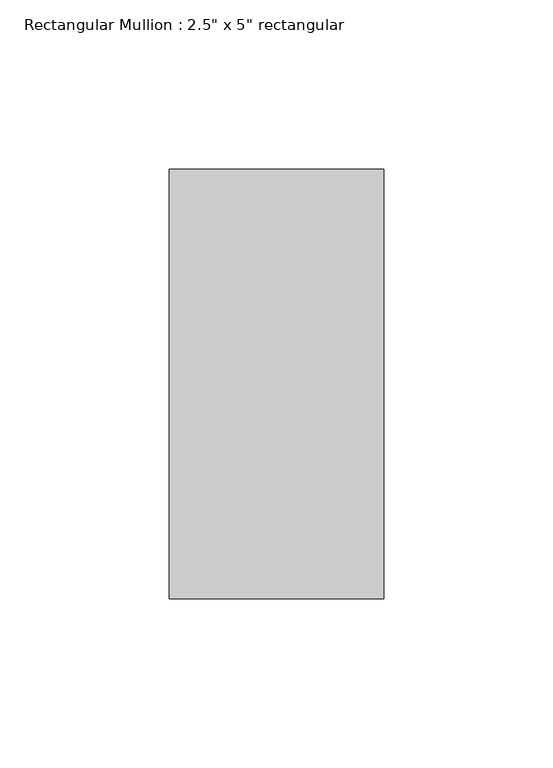
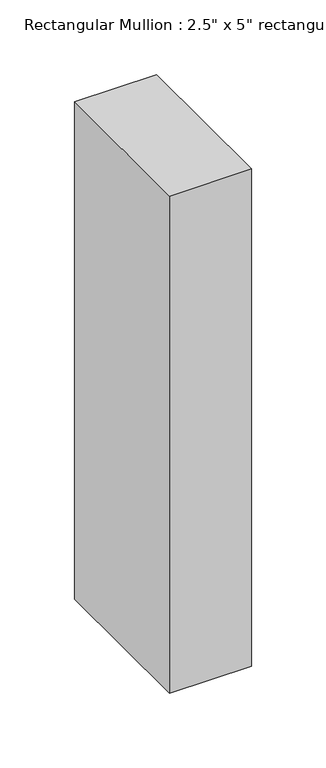
"""IFC4 building model written with IfcOpenShell, lengths in millimetres: member geometry."""

from ifc_helpers import new_model, si_unit, frame, origin, place, context, project, spatial, polyline, outline, extrude, source, transform, mapped, element, save


def member_90c805a2(model_context):
    return source(origin(), model_context, "Body", "SweptSolid", [
        extrude(outline(polyline([(31.75, 63.5), (31.75, -63.5), (-31.75, -63.5), (-31.75, 63.5), (31.75, 63.5)])), frame((0.0, 0.0, -406.4), z_axis=(0.0, 0.0, 1.0), x_axis=(1.0, 0.0, 0.0)), (0.0, 0.0, 1.0), 406.4),
    ])


if __name__ == "__main__":
    model = new_model("IFC4")
    model_context = context("Model", 3, world=origin())
    ifc_project = project(units=[si_unit("LENGTHUNIT", "METRE", prefix="MILLI")], contexts=[model_context])
    site = spatial("IfcSite", under=ifc_project)
    building = spatial("IfcBuilding", under=site)
    placement = place(None, origin())
    member_shape = member_90c805a2(model_context)
    element("IfcMember", 1, ObjectType="Rectangular Mullion : 2.5\" x 5\" rectangular", at=placement, inside=building, context=model_context, shape_type="MappedRepresentation", body=[
        mapped(member_shape, transform((0.0, 0.0, 0.0), x_axis=(1.0, 0.0, 0.0), y_axis=(0.0, 1.0, 0.0), z_axis=(0.0, 0.0, 1.0))),
    ])
    save(model, "model.ifc")

# Revit data of these elements
# Type "Rectangular Mullion : 2.5\" x 5\" rectangular"
#   built-in parameter 1007304 = 0.416667 (stored number, unit not read)
#   built-in parameter 1007301 = 0.104167 (stored number, unit not read)
#   built-in parameter 1007300 = 0.104167 (stored number, unit not read)
# Element 1 (IfcMember, "Rectangular Mullion : 2.5\" x 5\" rectangular")
#   Materials on its faces: "Door - Frame"
# Materials
#   "Door - Frame": colour RGB 118 70 51, transparency 0, Cost = 0
